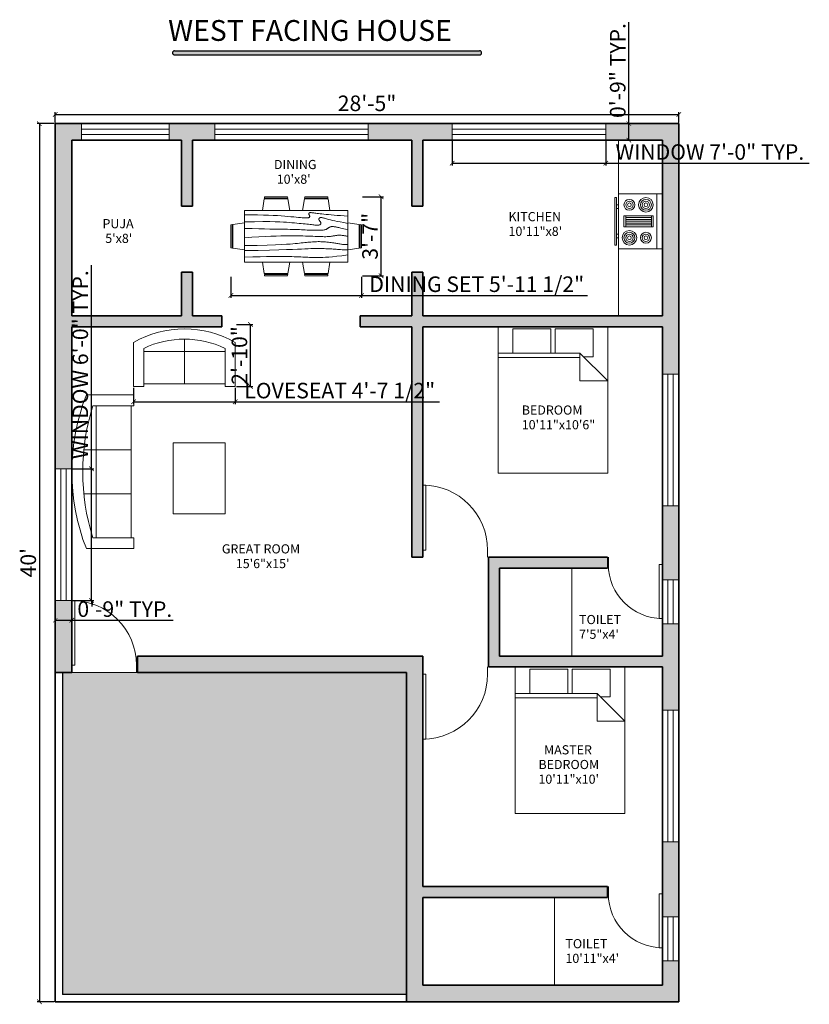
# Model space of a CAD drawing. Units: inches. Extents: x 3799 to 20199, y 1682 to 8087.
# Tile 30 of 30: x 19767 to 20199, y 6806 to 7344. Entities that reach past the tile are written whole.
import ezdxf

# ---------------------------------------------------------------- set-up
doc = ezdxf.new("R2010")
doc.units = ezdxf.units.IN
for name, color, linetype, lineweight in [('A-ANNO-DIMS', 2, 'Continuous', 18), ('A-ANNO-TITL', 7, 'Continuous', 25), ('A-AREA-IDEN', 7, 'Continuous', 18), ('A-DOOR', 3, 'Continuous', 18), ('A-EQPM', 9, 'Continuous', 18), ('A-FLOR-CASE', 32, 'Continuous', 18), ('A-FLOR-FIXT', 9, 'Continuous', 18), ('A-FURN', 8, 'Continuous', 18), ('A-GLAZ', 152, 'Continuous', 18), ('A-WALL', 7, 'Continuous', 35), ('A-WALL-PATT', 252, 'Continuous', 13), ('C-PROP', 7, 'Continuous', 25), ('L-PAVE', 253, 'Continuous', 13)]:
    doc.layers.add(name, color=color, linetype=linetype, lineweight=lineweight)
doc.styles.get("Standard").update_dxf_attribs({"font": 'arial.ttf'})
doc.dimstyles.new('ISO-25', dxfattribs={"dimtxt": 8.5, "dimasz": 2.5, "dimexe": 1.25, "dimexo": 0.625, "dimtad": 1, "dimdec": 0, "dimlunit": 3, "dimtxsty": 'Standard', "dimblk": 'ARCHTICK', "dimcen": 2.5, "dimadec": 0, "dimazin": 0, "dimtfac": 1, "dimtdec": 0, "dimtmove": 0, "dimatfit": 3, "dimfxl": 1, "dimarcsym": 0})

# ---------------------------------------------------------------- blocks, each defined once
blk = doc.blocks.new('*U49')
for p, q in [((0, 0), (0, -100)), ((900, 0), (900, -100))]:
    blk.add_line(p, q)
blk.add_lwpolyline([(0, 0), (0, 900), (43.75, 900), (43.75, 0)], close=True)
blk.add_arc((0, 0), 900, 0, 90)
blk = doc.blocks.new('*U215')
for p, q in [((0, 0), (0, 100)), ((900, 0), (900, 100))]:
    blk.add_line(p, q)
blk.add_lwpolyline([(0, 0), (0, -900), (43.75, -900), (43.75, 0)], close=True)
blk.add_arc((0, 0), 900, 270, 0)
blk = doc.blocks.new('*U216')
for p, q in [((-750, 0), (-750, 100)), ((0, 0), (0, 100))]:
    blk.add_line(p, q)
blk.add_lwpolyline([(0, 0), (0, -750), (-43.75, -750), (-43.75, 0)], close=True)
blk.add_arc((0, 0), 750, 180, 270)
blk = doc.blocks.new('Dining Set - 36 x 72 in.')
for p, q in [((-22, 27.5), (-22.1562, 26.50042)), ((-22, 27.5), (-6, 27.5)), ((-5.8437, 26.49966), (-6, 27.5)), ((6, 27.5), (5.8438, 26.50042)), ((6, 27.5), (22, 27.5)), ((22.1563, 26.49966), (22, 27.5)), ((-22.2343, 26.00059), (-23.4847, 17.99762)), ((-22.2304, 26), (-5.7608, 26)), ((-5.8416, 26.5), (-22.1534, 26.5)), ((-4.5152, 17.99762), (-5.7655, 25.99926)), ((5.7657, 26.00059), (4.5153, 17.99762)), ((5.7696, 26), (22.2392, 26)), ((22.1584, 26.5), (5.8466, 26.5)), ((23.4848, 17.99762), (22.2345, 25.99926)), ((36, 18), (-36, 18)), ((-36, 18), (-36, -18)), ((36, -18), (36, 18)), ((-45.5, 8), (-44.5004, 8.15617)), ((-45.5, 8), (-45.5, -8)), ((-44.5, -8.15843), (-44.5, 8.15338)), ((-44.0006, 8.23428), (-35.9976, 9.48474)), ((-44, 8.23041), (-44, -8.23915)), ((44.0006, 8.23428), (35.9976, 9.48474)), ((44, 8.23041), (44, -8.23915)), ((44.5, -8.15843), (44.5, 8.15338)), ((45.5, 8), (44.5005, 8.15617)), ((45.5, 8), (45.5, -8)), ((-44.4997, -8.15631), (-45.5, -8)), ((-35.9976, -9.48476), (-43.9993, -8.2345)), ((35.9976, -9.48476), (43.9993, -8.2345)), ((44.4997, -8.15631), (45.5, -8)), ((-36, -18), (36, -18)), ((-22.2343, -26.0006), (-23.4847, -17.99762)), ((-4.5152, -17.99762), (-5.7655, -25.99928)), ((5.7657, -26.0006), (4.5153, -17.99762)), ((23.4848, -17.99762), (22.2345, -25.99928)), ((-22.2304, -26), (-5.7608, -26)), ((-22, -27.5), (-22.1562, -26.50044)), ((-5.8416, -26.5), (-22.1534, -26.5)), ((-5.8437, -26.49967), (-6, -27.5)), ((5.7696, -26), (22.2392, -26)), ((6, -27.5), (5.8438, -26.50044)), ((22.1584, -26.5), (5.8466, -26.5)), ((22.1563, -26.49967), (22, -27.5)), ((-22, -27.5), (-6, -27.5)), ((6, -27.5), (22, -27.5))]:
    blk.add_line(p, q)
for points in [[(-36, 15), (-31.1772, 14.97754), (-26.8079, 14.91406), (-22.8538, 14.81543), (-19.276, 14.6875), (-16.0362, 14.53613), (-13.0957, 14.36718), (-10.4159, 14.18652), (-7.9583, 14), (-5.6904, 13.81315), (-3.6035, 13.63021), (-1.6954, 13.45508), (0.0365, 13.29166), (1.5945, 13.14388), (2.9811, 13.01562), (4.1988, 12.9108), (5.25, 12.83333), (6.1393, 12.78613), (6.8802, 12.76823), (7.4883, 12.77767), (7.9792, 12.8125), (8.3685, 12.87077), (8.6719, 12.95052), (8.9049, 13.0498), (9.0833, 13.16666), (9.2205, 13.29899), (9.3216, 13.44401), (9.3895, 13.59879), (9.4271, 13.76041), (9.4373, 13.92594), (9.4232, 14.09245), (9.3875, 14.257), (9.3333, 14.41666), (9.2638, 14.56917), (9.1836, 14.71484), (9.0975, 14.85465), (9.0104, 14.98958), (8.9272, 15.1206), (8.8529, 15.2487), (8.7922, 15.37483), (8.75, 15.5), (8.7305, 15.62467), (8.7344, 15.74739), (8.7617, 15.86621), (8.8125, 15.97916), (8.8867, 16.08431), (8.9844, 16.17968), (9.1055, 16.26334), (9.25, 16.33333), (9.4189, 16.38802), (9.6172, 16.42708), (9.8506, 16.45052), (10.125, 16.45833), (10.4463, 16.45052), (10.8203, 16.42708), (11.2529, 16.38802), (11.75, 16.33333), (12.3184, 16.26318), (12.9694, 16.17838), (13.7151, 16.07991), (14.5677, 15.96875), (15.5395, 15.84586), (16.6426, 15.71224), (17.8893, 15.56884), (19.2917, 15.41666), (20.859, 15.25667), (22.5879, 15.08984), (24.4721, 14.91715), (26.5052, 14.73958), (28.6809, 14.5581), (30.9929, 14.3737), (33.4347, 14.18733), (36, 14)], [(-36, 10), (-28.9766, 10.14274), (-23.1725, 10.20442), (-18.4241, 10.19775), (-14.5677, 10.13541), (-11.4399, 10.03011), (-8.877, 9.89453), (-6.7154, 9.74137), (-4.7917, 9.58333), (-2.9698, 9.43082), (-1.2246, 9.28515), (0.4415, 9.14534), (2.026, 9.01041), (3.5266, 8.87939), (4.9408, 8.7513), (6.266, 8.62516), (7.5, 8.5), (8.6411, 8.37549), (9.6914, 8.2539), (10.6538, 8.13818), (11.5312, 8.03125), (12.3267, 7.93603), (13.043, 7.85547), (13.6831, 7.79248), (14.25, 7.75), (14.7471, 7.7303), (15.1797, 7.73307), (15.5537, 7.75732), (15.875, 7.80208), (16.1494, 7.86637), (16.3828, 7.94922), (16.5811, 8.04964), (16.75, 8.16666), (16.8944, 8.29915), (17.0143, 8.44531), (17.1089, 8.60319), (17.1771, 8.77083), (17.218, 8.94629), (17.2305, 9.1276), (17.2137, 9.31282), (17.1667, 9.5), (17.0895, 9.6875), (16.987, 9.875), (16.8649, 10.0625), (16.7292, 10.25), (16.5856, 10.4375), (16.4401, 10.625), (16.2985, 10.8125), (16.1667, 11), (16.05, 11.18733), (15.9518, 11.3737), (15.8752, 11.5581), (15.8229, 11.73958), (15.798, 11.91715), (15.8034, 12.08984), (15.842, 12.25667), (15.9167, 12.41666), (16.0295, 12.56836), (16.1784, 12.70833), (16.3605, 12.83268), (16.5729, 12.9375), (16.8127, 13.01888), (17.0768, 13.07291), (17.3625, 13.0957), (17.6667, 13.08333), (17.9894, 13.03312), (18.3418, 12.94726), (18.7382, 12.82918), (19.1927, 12.68229), (19.7195, 12.51001), (20.3327, 12.31575), (21.0465, 12.10294), (21.875, 11.875), (22.8357, 11.63354), (23.959, 11.37304), (25.2786, 11.08618), (26.8282, 10.76562), (28.6414, 10.40405), (30.752, 9.99414), (33.1936, 9.52856), (36, 9)], [(-36, 5.5), (-30.7157, 5.3348), (-26.069, 5.20963), (-21.9946, 5.11767), (-18.4271, 5.05208), (-15.3009, 5.00602), (-12.5508, 4.97265), (-10.1112, 4.94515), (-7.9167, 4.91666), (-5.909, 4.88167), (-4.0586, 4.83984), (-2.3429, 4.79215), (-0.7396, 4.73958), (0.7739, 4.6831), (2.22, 4.6237), (3.6213, 4.56233), (5, 4.5), (6.373, 4.43782), (7.7344, 4.3776), (9.0723, 4.32129), (10.375, 4.27083), (11.6309, 4.22819), (12.8281, 4.19531), (13.9551, 4.17415), (15, 4.16666), (15.954, 4.17448), (16.819, 4.19791), (17.6001, 4.23698), (18.3021, 4.29166), (18.9299, 4.36198), (19.4883, 4.44791), (19.9823, 4.54948), (20.4167, 4.66666), (20.7969, 4.79899), (21.1302, 4.94401), (21.4245, 5.09879), (21.6875, 5.26041), (21.9271, 5.42594), (22.1511, 5.59245), (22.3672, 5.757), (22.5834, 5.91666), (22.8065, 6.06868), (23.0404, 6.21093), (23.2879, 6.34147), (23.5521, 6.45833), (23.8358, 6.55957), (24.142, 6.64323), (24.4735, 6.70735), (24.8334, 6.75), (25.2235, 6.76969), (25.642, 6.76692), (26.0858, 6.74267), (26.5521, 6.69791), (27.0379, 6.63362), (27.5404, 6.55078), (28.0565, 6.45036), (28.5834, 6.33333), (29.1242, 6.19987), (29.7071, 6.04687), (30.3661, 5.87044), (31.1354, 5.66666), (32.0493, 5.43164), (33.142, 5.16146), (34.4475, 4.85221), (36, 4.5)], [(-36, -1), (-30.7915, -0.6591), (-26.0195, -0.38216), (-21.6519, -0.16284), (-17.6563, 0.00521), (-14.0005, 0.12833), (-10.6523, 0.21289), (-7.5796, 0.26522), (-4.75, 0.29166), (-2.134, 0.29793), (0.2878, 0.28711), (2.5317, 0.26163), (4.6146, 0.22396), (6.5529, 0.17651), (8.3633, 0.12174), (10.0623, 0.06209), (11.6667, 0), (13.1899, -0.06201), (14.6341, -0.1211), (15.9982, -0.17432), (17.2813, -0.21875), (18.4823, -0.25147), (19.6003, -0.26953), (20.6343, -0.27002), (21.5834, -0.25), (22.4481, -0.20768), (23.2357, -0.14584), (23.9549, -0.06836), (24.6146, 0.02083), (25.2235, 0.11784), (25.7904, 0.21875), (26.3241, 0.31966), (26.8334, 0.41666), (27.3265, 0.50618), (27.8099, 0.58593), (28.2894, 0.65397), (28.7709, 0.70833), (29.2601, 0.74707), (29.763, 0.76823), (30.2855, 0.76985), (30.8334, 0.75), (31.4088, 0.70784), (31.9994, 0.64713), (32.589, 0.57275), (33.1615, 0.48958), (33.7008, 0.4025), (34.1908, 0.3164), (34.6153, 0.23616), (34.9584, 0.16666), (35.2099, 0.11165), (35.3848, 0.07031), (35.504, 0.04069), (35.5886, 0.02083), (35.6594, 0.00879), (35.7377, 0.0026), (35.8442, 0.00032), (36, 0)], [(-36, -6.5), (-27.1843, -6.31267), (-20.084, -6.1263), (-14.469, -5.9419), (-10.1094, -5.76042), (-6.7752, -5.58285), (-4.2363, -5.41016), (-2.2629, -5.24333), (-0.625, -5.08334), (0.8708, -4.93099), (2.2715, -4.78646), (3.5872, -4.64974), (4.8281, -4.52084), (6.0046, -4.39974), (7.127, -4.28646), (8.2053, -4.18099), (9.25, -4.08334), (10.2705, -3.99382), (11.2734, -3.91407), (12.2647, -3.84603), (13.25, -3.79167), (14.2354, -3.75293), (15.2266, -3.73177), (16.2295, -3.73015), (17.25, -3.75), (18.2912, -3.79248), (19.3451, -3.85547), (20.4009, -3.93604), (21.4479, -4.03125), (22.4754, -4.13819), (23.4727, -4.25391), (24.4289, -4.37549), (25.3334, -4.5), (26.1785, -4.62492), (26.9694, -4.74935), (27.7145, -4.87281), (28.4219, -4.99479), (29.1, -5.11483), (29.7572, -5.23242), (30.4016, -5.34709), (31.0417, -5.45834), (31.6837, -5.56437), (32.3262, -5.65821), (32.9658, -5.73153), (33.599, -5.77604), (34.2224, -5.78345), (34.8327, -5.74545), (35.4264, -5.65373), (36, -5.5)], [(-36, -10), (-26.4022, -9.81299), (-18.4675, -9.62891), (-11.9839, -9.45069), (-6.7396, -9.28125), (-2.5226, -9.12354), (0.8789, -8.98047), (3.6769, -8.85498), (6.0833, -8.75), (8.2767, -8.66765), (10.3021, -8.60677), (12.1712, -8.56543), (13.8958, -8.54167), (15.4876, -8.53353), (16.9583, -8.53907), (18.3197, -8.55632), (19.5834, -8.58334), (20.7616, -8.61841), (21.8685, -8.66081), (22.9188, -8.71004), (23.9271, -8.76563), (24.9081, -8.82707), (25.8763, -8.89388), (26.8465, -8.96558), (27.8334, -9.04167), (28.8474, -9.12118), (29.8828, -9.20117), (30.93, -9.27824), (31.9792, -9.34896), (33.0205, -9.40991), (34.0443, -9.45768), (35.0407, -9.48885), (36, -9.5)], [(-36, -14.5), (-30.0881, -14.33513), (-25.0332, -14.21224), (-20.7312, -14.12647), (-17.0781, -14.07292), (-13.97, -14.04671), (-11.3027, -14.04297), (-8.9724, -14.05681), (-6.875, -14.08334), (-4.9224, -14.11833), (-3.0905, -14.16016), (-1.3709, -14.20785), (0.2448, -14.26042), (1.7647, -14.3169), (3.1973, -14.3763), (4.5507, -14.43767), (5.8333, -14.5), (7.0554, -14.5621), (8.235, -14.62175), (9.3922, -14.67652), (10.5469, -14.72396), (11.7192, -14.76164), (12.929, -14.78711), (14.1965, -14.79794), (15.5417, -14.79167), (16.9933, -14.76424), (18.6152, -14.70508), (20.4804, -14.60197), (22.6615, -14.44271), (25.2312, -14.21509), (28.2624, -13.9069), (31.8277, -13.50594), (36, -13)]]:
    blk.add_lwpolyline(points)
blk = doc.blocks.new('Bed - Queen')
for p, q in [((0, -80.00003), (0, 0)), ((0, 0), (59.99999, 0)), ((59.99999, 0), (59.99999, -80.00003)), ((7.99999, -1.2), (28.79998, -1.2)), ((7.99999, -14.4), (7.99999, -1.2)), ((28.79998, -1.2), (28.79998, -14.4)), ((31.19999, -1.2), (51.99999, -1.2)), ((31.19999, -14.4), (31.19999, -1.2)), ((51.99999, -1.2), (51.99999, -16.4)), ((0, -14.4), (44.8, -14.4)), ((59.99999, -29.6), (44.8, -14.4)), ((44.8, -14.4), (44.8, -29.6)), ((44.8, -16.8), (0, -16.8)), ((51.99999, -16.4), (46.79936, -16.4)), ((44.8, -29.6), (59.99999, -29.6)), ((59.99999, -80.00003), (0, -80.00003))]:
    blk.add_line(p, q)
blk = doc.blocks.new('Range-Oven - 30 in top')
for p, q in [((0, -3), (30, -3)), ((12, -6), (18, -6)), ((13, -20), (13, -6)), ((14, -6), (14, -20)), ((15, -20), (15, -6)), ((16, -6), (16, -20)), ((17, -20), (17, -6)), ((18, -20), (12, -20)), ((6, -24), (6, -25)), ((8, -25), (8, -24)), ((22, -25), (22, -24)), ((24, -24), (24, -25))]:
    blk.add_line(p, q)
for points in [[(0, -24), (0, 0), (30, 0), (30, -24)], [(12, -21), (12, -5), (18, -5), (18, -21)], [(2, -26), (2, -25), (28, -25), (28, -26)]]:
    blk.add_lwpolyline(points, close=True)
for centre, radius in [((6, -9), 4), ((6, -9), 3), ((6, -9), 2), ((6, -9), 1), ((24, -9), 3), ((24, -9), 2), ((24, -9), 1), ((6, -18), 3), ((6, -18), 2), ((24, -18), 4), ((24, -18), 3), ((24, -18), 2), ((6, -18), 1), ((24, -18), 1)]:
    blk.add_circle(centre, radius)
blk = doc.blocks.new('Sofa - Roundback 7 ft.')
for p, q in [((-12.00002, -32.4421), (-12.00003, -6.5971)), ((11.99997, -32.4421), (11.99998, -6.5971)), ((-36.000027, -34), (-36.000027, -11.4696)), ((-35.999844, -13.3819), (35.9998, -13.3819)), ((35.99998, -34), (35.99998, -11.4696)), ((-36.000027, -32.4421), (35.99998, -32.4421))]:
    blk.add_line(p, q)
for points in [[(-36.000027, -34), (-42.000027, -34), (-42.000027, -8)], [(41.99998, -8), (41.99998, -34), (35.99998, -34)]]:
    blk.add_lwpolyline(points)
for centre, radius, start, end in [((0, -114.25), 114.25, 68.43141, 111.5686), ((-0.00001, -127.1968), 121.1968, 72.72033, 107.2797)]:
    blk.add_arc(centre, radius, start, end)
blk = doc.blocks.new('Sofa - Roundback Loveseat 5 ft.')
for p, q in [((-24, -33.99998), (-24, -11.46958)), ((0, -32.44198), (0, -5.99998)), ((24.00004, -33.99998), (24.00004, -11.46958)), ((-23.9998, -13.38178), (23.99986, -13.38178)), ((-24, -32.44198), (24.00004, -32.44198))]:
    blk.add_line(p, q)
for points in [[(-24, -33.99998), (-30, -33.99998), (-30, -7.99998)], [(30.00004, -7.99998), (30.00004, -33.99998), (24.00004, -33.99998)]]:
    blk.add_lwpolyline(points)
for centre, radius, start, end in [((0, -60.24998), 60.24998, 60.13715, 119.8628), ((0, -61.38438), 55.38444, 64.32083, 115.6792)]:
    blk.add_arc(centre, radius, start, end)
blk = doc.blocks.new('_ArchTick')
at = {"color": 0, "linetype": 'ByBlock', "const_width": 0.15}
blk.add_lwpolyline([(-0.5, -0.5), (0.5, 0.5)], dxfattribs=at)
blk = doc.blocks.new('*D217')
at = {"layer": 'A-ANNO-DIMS', "color": 0, "lineweight": -2, "transparency": 16777216}
for p, q in [((19786.54, 7287.57), (19786.54, 7293.26)), ((20127.54, 7287.57), (20127.54, 7293.26)), ((19786.54, 7292.01), (20127.54, 7292.01))]:
    blk.add_line(p, q, dxfattribs=at)
at = {"layer": 'Defpoints', "color": 0, "transparency": 16777216}
for p in [(20127.54, 7292.01), (19786.54, 7286.95), (20127.54, 7286.95)]:
    blk.add_point(p, dxfattribs=at)
at = {"layer": 'A-ANNO-DIMS', "color": 0, "lineweight": -2, "transparency": 16777216, "xscale": 2.5, "yscale": 2.5, "zscale": 2.5, "rotation": 180}
blk.add_blockref('_ArchTick', (19786.54, 7292.01), dxfattribs=at)
at = {"layer": 'A-ANNO-DIMS', "color": 0, "lineweight": -2, "transparency": 16777216, "xscale": 2.5, "yscale": 2.5, "zscale": 2.5}
blk.add_blockref('_ArchTick', (20127.54, 7292.01), dxfattribs=at)
at = {"layer": 'A-ANNO-DIMS', "color": 0, "transparency": 16777216, "insert": (19957.04, 7296.97), "char_height": 8.5, "attachment_point": 5}
blk.add_mtext('28\'-5"', dxfattribs=at)
blk = doc.blocks.new('*D218')
at = {"layer": 'A-ANNO-DIMS', "color": 0, "lineweight": -2, "transparency": 16777216}
for p, q in [((19785.92, 7286.95), (19776.58, 7286.95)), ((19777.83, 7286.95), (19777.83, 6806.95)), ((19785.92, 6806.95), (19776.58, 6806.95))]:
    blk.add_line(p, q, dxfattribs=at)
at = {"layer": 'Defpoints', "color": 0, "transparency": 16777216}
for p in [(19786.54, 7286.95), (19777.83, 6806.95), (19786.54, 6806.95)]:
    blk.add_point(p, dxfattribs=at)
at = {"layer": 'A-ANNO-DIMS', "color": 0, "lineweight": -2, "transparency": 16777216, "xscale": 2.5, "yscale": 2.5, "zscale": 2.5}
for p, rotation in [((19777.83, 7286.95), 90), ((19777.83, 6806.95), 270)]:
    blk.add_blockref('_ArchTick', p, dxfattribs=dict(at, rotation=rotation))
at = {"layer": 'A-ANNO-DIMS', "color": 0, "transparency": 16777216, "insert": (19772.87, 7046.95), "char_height": 8.5, "attachment_point": 5, "rotation": 90}
blk.add_mtext("40'", dxfattribs=at)
blk = doc.blocks.new('WIN-24IN-9IN-FRAME')
for p, q in [((0, 24), (9, 24)), ((3, 0), (3, 24)), ((6, 0), (6, 24)), ((0, 0), (9, 0))]:
    blk.add_line(p, q)
blk = doc.blocks.new('WIN-48IN-9IN-FRAME')
for p, q in [((0, 0), (0, 9)), ((48, 6), (0, 6)), ((48, 0), (48, 9)), ((48, 3), (0, 3))]:
    blk.add_line(p, q)
blk = doc.blocks.new('WIN-84IN-9IN-FRAME')
for p, q in [((0, 0), (0, 9)), ((0, 6), (84, 6)), ((84, 0), (84, 9)), ((0, 3), (84, 3))]:
    blk.add_line(p, q)
blk = doc.blocks.new('WIN-72IN-9IN-FRAME')
for p, q in [((0, 72), (9, 72)), ((3, 72), (3, 0)), ((6, 72), (6, 0)), ((0, 0), (9, 0))]:
    blk.add_line(p, q)
blk = doc.blocks.new('*D282')
at = {"layer": 'A-ANNO-DIMS', "color": 0, "lineweight": -2, "transparency": 16777216}
for p, q in [((19829.38, 7142.62), (19829.38, 7133.66)), ((19884.97, 7142.62), (19884.97, 7133.66)), ((19829.38, 7134.91), (19884.97, 7134.91)), ((19884.97, 7134.91), (19996.73, 7134.91))]:
    blk.add_line(p, q, dxfattribs=at)
at = {"layer": 'Defpoints', "color": 0, "transparency": 16777216}
for p in [(19829.38, 7143.25), (19884.97, 7143.25), (19884.97, 7134.91)]:
    blk.add_point(p, dxfattribs=at)
at = {"layer": 'A-ANNO-DIMS', "color": 0, "lineweight": -2, "transparency": 16777216, "xscale": 2.5, "yscale": 2.5, "zscale": 2.5, "rotation": 180}
blk.add_blockref('_ArchTick', (19829.38, 7134.91), dxfattribs=at)
at = {"layer": 'A-ANNO-DIMS', "color": 0, "lineweight": -2, "transparency": 16777216, "xscale": 2.5, "yscale": 2.5, "zscale": 2.5}
blk.add_blockref('_ArchTick', (19884.97, 7134.91), dxfattribs=at)
at = {"layer": 'A-ANNO-DIMS', "color": 0, "transparency": 16777216, "insert": (19942.1, 7139.93), "char_height": 8.5, "attachment_point": 5}
blk.add_mtext('LOVESEAT 4\'-7 1/2"', dxfattribs=at)
blk = doc.blocks.new('*D283')
at = {"layer": 'A-ANNO-DIMS', "color": 0, "lineweight": -2, "transparency": 16777216}
for p, q in [((19885.59, 7177.21), (19894.55, 7177.21)), ((19893.3, 7143.25), (19893.3, 7177.21)), ((19885.59, 7143.25), (19894.55, 7143.25))]:
    blk.add_line(p, q, dxfattribs=at)
at = {"layer": 'Defpoints', "color": 0, "transparency": 16777216}
for p in [(19884.97, 7177.21), (19893.3, 7177.21), (19884.97, 7143.25)]:
    blk.add_point(p, dxfattribs=at)
at = {"layer": 'A-ANNO-DIMS', "color": 0, "lineweight": -2, "transparency": 16777216, "xscale": 2.5, "yscale": 2.5, "zscale": 2.5}
for p, rotation in [((19893.3, 7177.21), 90), ((19893.3, 7143.25), 270)]:
    blk.add_blockref('_ArchTick', p, dxfattribs=dict(at, rotation=rotation))
at = {"layer": 'A-ANNO-DIMS', "color": 0, "transparency": 16777216, "insert": (19888.34, 7160.23), "char_height": 8.5, "attachment_point": 5, "rotation": 90}
blk.add_mtext('2\'-10"', dxfattribs=at)
blk = doc.blocks.new('*D296')
at = {"layer": 'A-ANNO-DIMS', "color": 0, "lineweight": -2, "transparency": 16777216}
for p, q in [((19882.55, 7203.16), (19882.55, 7191.82)), ((19954, 7203.16), (19954, 7191.82)), ((19882.55, 7193.07), (19954, 7193.07)), ((19954, 7193.07), (20077.58, 7193.07))]:
    blk.add_line(p, q, dxfattribs=at)
at = {"layer": 'Defpoints', "color": 0, "transparency": 16777216}
for p in [(19882.55, 7203.78), (19954, 7203.78), (19954, 7193.07)]:
    blk.add_point(p, dxfattribs=at)
at = {"layer": 'A-ANNO-DIMS', "color": 0, "lineweight": -2, "transparency": 16777216, "xscale": 2.5, "yscale": 2.5, "zscale": 2.5, "rotation": 180}
blk.add_blockref('_ArchTick', (19882.55, 7193.07), dxfattribs=at)
at = {"layer": 'A-ANNO-DIMS', "color": 0, "lineweight": -2, "transparency": 16777216, "xscale": 2.5, "yscale": 2.5, "zscale": 2.5}
blk.add_blockref('_ArchTick', (19954, 7193.07), dxfattribs=at)
at = {"layer": 'A-ANNO-DIMS', "color": 0, "transparency": 16777216, "insert": (20017.04, 7198.09), "char_height": 8.5, "attachment_point": 5}
blk.add_mtext('DINING SET 5\'-11 1/2"', dxfattribs=at)
blk = doc.blocks.new('*D297')
at = {"layer": 'A-ANNO-DIMS', "color": 0, "lineweight": -2, "transparency": 16777216}
for p, q in [((19954.62, 7246.97), (19965.97, 7246.97)), ((19964.72, 7203.78), (19964.72, 7246.97)), ((19954.62, 7203.78), (19965.97, 7203.78))]:
    blk.add_line(p, q, dxfattribs=at)
at = {"layer": 'Defpoints', "color": 0, "transparency": 16777216}
for p in [(19954, 7246.97), (19964.72, 7246.97), (19954, 7203.78)]:
    blk.add_point(p, dxfattribs=at)
at = {"layer": 'A-ANNO-DIMS', "color": 0, "lineweight": -2, "transparency": 16777216, "xscale": 2.5, "yscale": 2.5, "zscale": 2.5}
for p, rotation in [((19964.72, 7246.97), 90), ((19964.72, 7203.78), 270)]:
    blk.add_blockref('_ArchTick', p, dxfattribs=dict(at, rotation=rotation))
at = {"layer": 'A-ANNO-DIMS', "color": 0, "transparency": 16777216, "insert": (19959.75, 7225.38), "char_height": 8.5, "attachment_point": 5, "rotation": 90}
blk.add_mtext('3\'-7"', dxfattribs=at)
blk = doc.blocks.new('*D328')
at = {"layer": 'A-ANNO-DIMS', "color": 0, "lineweight": -2, "transparency": 16777216}
for p, q in [((19806.34, 7098.32), (19806.34, 7209.63)), ((19796.17, 7098.32), (19807.59, 7098.32)), ((19806.34, 7026.32), (19806.34, 7098.32)), ((19796.17, 7026.32), (19807.59, 7026.32))]:
    blk.add_line(p, q, dxfattribs=at)
at = {"layer": 'Defpoints', "color": 0, "transparency": 16777216}
for p in [(19795.54, 7098.32), (19806.34, 7098.32), (19795.54, 7026.32)]:
    blk.add_point(p, dxfattribs=at)
at = {"layer": 'A-ANNO-DIMS', "color": 0, "lineweight": -2, "transparency": 16777216, "xscale": 2.5, "yscale": 2.5, "zscale": 2.5}
for p, rotation in [((19806.34, 7098.32), 90), ((19806.34, 7026.32), 270)]:
    blk.add_blockref('_ArchTick', p, dxfattribs=dict(at, rotation=rotation))
at = {"layer": 'A-ANNO-DIMS', "color": 0, "transparency": 16777216, "insert": (19801.32, 7155.22), "char_height": 8.5, "attachment_point": 5, "rotation": 90}
blk.add_mtext('WINDOW 6\'-0" TYP.', dxfattribs=at)
blk = doc.blocks.new('*D329')
at = {"layer": 'A-ANNO-DIMS', "color": 0, "lineweight": -2, "transparency": 16777216}
for p, q in [((19786.54, 7025.69), (19786.54, 7014.27)), ((19795.54, 7025.69), (19795.54, 7014.27)), ((19786.54, 7015.52), (19795.54, 7015.52)), ((19795.54, 7015.52), (19851.1, 7015.52))]:
    blk.add_line(p, q, dxfattribs=at)
at = {"layer": 'Defpoints', "color": 0, "transparency": 16777216}
for p in [(19786.54, 7026.32), (19795.54, 7026.32), (19795.54, 7015.52)]:
    blk.add_point(p, dxfattribs=at)
at = {"layer": 'A-ANNO-DIMS', "color": 0, "lineweight": -2, "transparency": 16777216, "xscale": 2.5, "yscale": 2.5, "zscale": 2.5, "rotation": 180}
blk.add_blockref('_ArchTick', (19786.54, 7015.52), dxfattribs=at)
at = {"layer": 'A-ANNO-DIMS', "color": 0, "lineweight": -2, "transparency": 16777216, "xscale": 2.5, "yscale": 2.5, "zscale": 2.5}
blk.add_blockref('_ArchTick', (19795.54, 7015.52), dxfattribs=at)
at = {"layer": 'A-ANNO-DIMS', "color": 0, "transparency": 16777216, "insert": (19824.57, 7020.48), "char_height": 8.5, "attachment_point": 5}
blk.add_mtext('0\'-9" TYP.', dxfattribs=at)
blk = doc.blocks.new('*D340')
at = {"layer": 'A-ANNO-DIMS', "color": 0, "lineweight": -2, "transparency": 16777216}
for p, q in [((20003.6, 7277.32), (20003.6, 7264.1)), ((20087.6, 7277.32), (20087.6, 7264.1)), ((20003.6, 7265.35), (20087.6, 7265.35)), ((20087.6, 7265.35), (20198.91, 7265.35))]:
    blk.add_line(p, q, dxfattribs=at)
at = {"layer": 'Defpoints', "color": 0, "transparency": 16777216}
for p in [(20003.6, 7277.95), (20087.6, 7277.95), (20087.6, 7265.35)]:
    blk.add_point(p, dxfattribs=at)
at = {"layer": 'A-ANNO-DIMS', "color": 0, "lineweight": -2, "transparency": 16777216, "xscale": 2.5, "yscale": 2.5, "zscale": 2.5, "rotation": 180}
blk.add_blockref('_ArchTick', (20003.6, 7265.35), dxfattribs=at)
at = {"layer": 'A-ANNO-DIMS', "color": 0, "lineweight": -2, "transparency": 16777216, "xscale": 2.5, "yscale": 2.5, "zscale": 2.5}
blk.add_blockref('_ArchTick', (20087.6, 7265.35), dxfattribs=at)
at = {"layer": 'A-ANNO-DIMS', "color": 0, "transparency": 16777216, "insert": (20144.51, 7270.37), "char_height": 8.5, "attachment_point": 5}
blk.add_mtext('WINDOW 7\'-0" TYP.', dxfattribs=at)
blk = doc.blocks.new('*D341')
at = {"layer": 'A-ANNO-DIMS', "color": 0, "lineweight": -2, "transparency": 16777216}
for p, q in [((20100.2, 7286.95), (20100.2, 7342.51)), ((20088.23, 7286.95), (20101.45, 7286.95)), ((20100.2, 7277.95), (20100.2, 7286.95)), ((20088.23, 7277.95), (20101.45, 7277.95))]:
    blk.add_line(p, q, dxfattribs=at)
at = {"layer": 'Defpoints', "color": 0, "transparency": 16777216}
for p in [(20087.6, 7286.95), (20100.2, 7286.95), (20087.6, 7277.95)]:
    blk.add_point(p, dxfattribs=at)
at = {"layer": 'A-ANNO-DIMS', "color": 0, "lineweight": -2, "transparency": 16777216, "xscale": 2.5, "yscale": 2.5, "zscale": 2.5}
for p, rotation in [((20100.2, 7286.95), 90), ((20100.2, 7277.95), 270)]:
    blk.add_blockref('_ArchTick', p, dxfattribs=dict(at, rotation=rotation))
at = {"layer": 'A-ANNO-DIMS', "color": 0, "transparency": 16777216, "insert": (20095.24, 7315.98), "char_height": 8.5, "attachment_point": 5, "rotation": 90}
blk.add_mtext('0\'-9" TYP.', dxfattribs=at)

msp = doc.modelspace()

# ---------------------------------------------------------------- hatches: boundary and pattern name
at = {"layer": 'A-ANNO-TITL'}
h = msp.add_hatch(color=256, dxfattribs=at)
h.dxf.hatch_style = 1
h.paths.add_polyline_path([(20018.56, 7326.79), (19851.73, 7326.79, 1), (19851.73, 7324.51), (20018.56, 7324.51, 1)])
at = {"layer": 'A-WALL-PATT'}
h = msp.add_hatch(color=256, dxfattribs=at)
h.dxf.hatch_style = 1
h.paths.add_polyline_path([(19795.54, 7277.95), (19800.83, 7277.95), (19800.83, 7286.95), (19786.54, 7286.95), (19786.54, 7098.32), (19795.54, 7098.32), (19795.54, 7175.95), (19877.69, 7175.95), (19877.69, 7181.95), (19861.54, 7181.95), (19861.54, 7205.82), (19855.54, 7205.82), (19855.54, 7181.95), (19795.54, 7181.95)])
h.paths.add_polyline_path([(19873.75, 7286.95), (19848.83, 7286.95), (19848.83, 7277.95), (19855.54, 7277.95), (19855.54, 7241.82), (19861.54, 7241.82), (19861.54, 7277.95), (19873.75, 7277.95)], flags=17)
h.paths.add_polyline_path([(20003.6, 7286.95), (19957.75, 7286.95), (19957.75, 7277.95), (19981.54, 7277.95), (19981.54, 7241.82), (19987.54, 7241.82), (19987.54, 7277.95), (20003.6, 7277.95)], flags=17)
h.paths.add_polyline_path([(20127.54, 7286.95), (20087.6, 7286.95), (20087.6, 7277.95), (20118.54, 7277.95), (20118.54, 7181.95), (19987.54, 7181.95), (19987.54, 7205.82), (19981.54, 7205.82), (19981.54, 7181.95), (19953.3, 7181.95), (19953.3, 7175.95), (19981.54, 7175.95), (19981.54, 7049.95), (19987.54, 7049.95), (19987.54, 7175.95), (20118.54, 7175.95), (20118.54, 7149.99), (20127.54, 7149.99)])
h.paths.add_polyline_path([(20127.54, 7077.99), (20118.54, 7077.99), (20118.54, 7049.95), (20118.54, 7037.51), (20127.54, 7037.51)])
h.paths.add_polyline_path([(20127.54, 7013.51), (20118.54, 7013.51), (20118.54, 6995.95), (20029.54, 6995.95), (20029.54, 7043.95), (20088.54, 7043.95), (20088.54, 7049.95), (20023.54, 7049.95), (20023.54, 7043.95), (20023.54, 6989.95), (20118.54, 6989.95), (20118.54, 6966.36), (20127.54, 6966.36)])
h.paths.add_polyline_path([(20127.54, 6894.36), (20118.54, 6894.36), (20118.54, 6853.34), (20127.54, 6853.34)], flags=17)
h.paths.add_polyline_path([(20088.54, 6869.95), (19987.54, 6869.95), (19987.54, 6995.95), (19831.54, 6995.95), (19831.54, 6986.95), (19978.54, 6986.95), (19978.54, 6806.95), (20127.54, 6806.95), (20127.54, 6829.34), (20118.54, 6829.34), (20118.54, 6815.95), (19987.54, 6815.95), (19987.54, 6863.95), (20088.54, 6863.95)])
h.paths.add_polyline_path([(19795.54, 7026.32), (19786.54, 7026.32), (19786.54, 6986.95), (19795.54, 6986.95)])
at = {"layer": 'L-PAVE'}
h = msp.add_hatch(color=256, dxfattribs=at)
h.dxf.hatch_style = 1
h.paths.add_polyline_path([(19978.54, 6986.95), (19831.54, 6986.95), (19795.54, 6986.95), (19790.54, 6986.95), (19790.54, 6810.95), (19978.54, 6810.95)])

# ---------------------------------------------------------------- linework, layer by layer
at = {"layer": 'A-ANNO-TITL'}
for p, q in [((19851.73, 7326.79), (20018.56, 7326.79)), ((19851.73, 7324.51), (20018.56, 7324.51))]:
    msp.add_line(p, q, dxfattribs=at)
for centre, start, end in [((19851.73, 7325.65), 90, 270), ((20018.56, 7325.65), 270, 90)]:
    msp.add_arc(centre, 1.14, start, end, dxfattribs=at)
at = {"layer": 'A-DOOR'}
msp.add_line((19795.54, 6986.95), (19831.54, 6986.95), dxfattribs=at)
at = {"layer": 'A-FLOR-CASE'}
msp.add_line((20094.54, 7277.95), (20094.54, 7181.95), dxfattribs=at)
at = {"layer": 'A-FLOR-FIXT'}
for p, q in [((20069.05, 7043.95), (20069.05, 6995.95)), ((20059.51, 6863.95), (20059.51, 6815.95))]:
    msp.add_line(p, q, dxfattribs=at)
at = {"layer": 'A-FURN'}
msp.add_lwpolyline([(19851.07, 7112.49), (19879.43, 7112.49), (19879.43, 7073.72), (19851.07, 7073.72)], close=True, dxfattribs=at)
at = {"layer": 'A-WALL'}
for p, q in [((19786.54, 6986.95), (19786.54, 7286.95)), ((19786.54, 7286.95), (20127.54, 7286.95)), ((20127.54, 7286.95), (20127.54, 6806.95)), ((19795.54, 7277.95), (19855.54, 7277.95)), ((19795.54, 7181.95), (19795.54, 7277.95)), ((19855.54, 7241.82), (19855.54, 7277.95)), ((19861.54, 7277.95), (19981.54, 7277.95)), ((19861.54, 7241.82), (19861.54, 7277.95)), ((19981.54, 7241.82), (19981.54, 7277.95)), ((19987.54, 7277.95), (20118.54, 7277.95)), ((19987.54, 7241.82), (19987.54, 7277.95)), ((20118.54, 7277.95), (20118.54, 7181.95)), ((19855.54, 7241.82), (19861.54, 7241.82)), ((19981.54, 7241.82), (19987.54, 7241.82)), ((19855.54, 7181.95), (19855.54, 7205.82)), ((19855.54, 7205.82), (19861.54, 7205.82)), ((19861.54, 7181.95), (19861.54, 7205.82)), ((19981.54, 7181.95), (19981.54, 7205.82)), ((19981.54, 7205.82), (19987.54, 7205.82)), ((19987.54, 7181.95), (19987.54, 7205.82)), ((19795.54, 7181.95), (19855.54, 7181.95)), ((19861.54, 7181.95), (19877.69, 7181.95)), ((19877.69, 7181.95), (19877.69, 7175.95)), ((19953.3, 7181.95), (19981.54, 7181.95)), ((19953.3, 7181.95), (19953.3, 7175.95)), ((19987.54, 7181.95), (20118.54, 7181.95)), ((19795.54, 6986.95), (19795.54, 7175.95)), ((19795.54, 7175.95), (19877.69, 7175.95)), ((19953.3, 7175.95), (19981.54, 7175.95)), ((19981.54, 7049.95), (19981.54, 7175.95)), ((19987.54, 7175.95), (20118.54, 7175.95)), ((19987.54, 7049.95), (19987.54, 7175.95)), ((20118.54, 7175.95), (20118.54, 7049.95)), ((19987.54, 7049.95), (19981.54, 7049.95)), ((20023.54, 7049.95), (20088.54, 7049.95)), ((20023.54, 7043.95), (20023.54, 7049.95)), ((20118.54, 7049.95), (20118.54, 6995.95)), ((20023.54, 7043.95), (20023.54, 6989.95)), ((20029.54, 7043.95), (20029.54, 6995.95)), ((20029.54, 7043.95), (20088.54, 7043.95)), ((19831.54, 6995.95), (19987.54, 6995.95)), ((19831.54, 6986.95), (19831.54, 6995.95)), ((19987.54, 6869.95), (19987.54, 6995.95)), ((20029.54, 6995.95), (20118.54, 6995.95)), ((19786.54, 6986.95), (19795.54, 6986.95)), ((19786.54, 6986.95), (19786.54, 6806.95)), ((19831.54, 6986.95), (19978.54, 6986.95)), ((19978.54, 6806.95), (19978.54, 6986.95)), ((20023.54, 6989.95), (20118.54, 6989.95)), ((20118.54, 6989.95), (20118.54, 6815.95)), ((19987.54, 6869.95), (20088.54, 6869.95)), ((20088.54, 6869.95), (20088.54, 6863.95)), ((19987.54, 6815.95), (19987.54, 6863.95)), ((19987.54, 6863.95), (20088.54, 6863.95)), ((20118.54, 6815.95), (19987.54, 6815.95)), ((20127.54, 6806.95), (19786.54, 6806.95))]:
    msp.add_line(p, q, dxfattribs=at)
at = {"layer": 'C-PROP'}
for p, q in [((20088.54, 7049.95), (20088.54, 7043.95)), ((19790.54, 6986.95), (19790.54, 6810.95)), ((19978.54, 6810.95), (19790.54, 6810.95))]:
    msp.add_line(p, q, dxfattribs=at)

# ---------------------------------------------------------------- block references
at = {"layer": 'A-DOOR', "xscale": 0.0393700787401575, "yscale": 0.0393700787401575, "zscale": 0.0393700787401575}
for name, p in [('*U49', (19987.54, 7053.88)), ('*U216', (20118.54, 7046.01)), ('*U49', (19795.54, 6990.88)), ('*U215', (19987.54, 6986.01)), ('*U216', (20118.54, 6866.01))]:
    msp.add_blockref(name, p, dxfattribs=at)
at = {"layer": 'A-EQPM', "rotation": 270}
msp.add_blockref('Range-Oven - 30 in top', (20118.54, 7248.58), dxfattribs=at)
at = {"layer": 'A-FURN'}
for name, p, xscale, yscale, zscale in [('Dining Set - 36 x 72 in.', (19918.27, 7225.38), 0.7851969363924316, 0.7851969363924316, 0.7851969363924316), ('Sofa - Roundback Loveseat 5 ft.', (19857.17, 7174.74), 0.9264126650425815, 0.9264126650425815, 0.9264126650425815)]:
    msp.add_blockref(name, p, dxfattribs=dict(at, xscale=xscale, yscale=yscale, zscale=zscale))
for p in [(20028.69, 7175.95), (20038.01, 6989.95)]:
    msp.add_blockref('Bed - Queen', p, dxfattribs=at)
at = {"layer": 'A-FURN', "rotation": 90}
msp.add_blockref('Sofa - Roundback 7 ft.', (19795.57, 7096.63), dxfattribs=at)
at = {"layer": 'A-GLAZ'}
for name, p in [('WIN-48IN-9IN-FRAME', (19800.83, 7277.95)), ('WIN-84IN-9IN-FRAME', (19873.74, 7277.95)), ('WIN-84IN-9IN-FRAME', (20003.6, 7277.95)), ('WIN-72IN-9IN-FRAME', (20118.54, 7077.99)), ('WIN-72IN-9IN-FRAME', (19786.54, 7026.32)), ('WIN-24IN-9IN-FRAME', (20118.54, 7013.51)), ('WIN-72IN-9IN-FRAME', (20118.54, 6894.36)), ('WIN-24IN-9IN-FRAME', (20118.54, 6829.34))]:
    msp.add_blockref(name, p, dxfattribs=at)

# ---------------------------------------------------------------- texts
at = {"layer": 'A-ANNO-TITL'}
msp.add_text('WEST FACING HOUSE', height=11.3809, rotation=0.0014, dxfattribs=at).set_placement((19848.28, 7332.19))
at = {"layer": 'A-AREA-IDEN'}
for s, p in [('DINING', (19906.13, 7262.12)), (" 10'x8'", (19906.13, 7254.09)), ('PUJA', (19812.35, 7229.79)), ('KITCHEN', (20034.4, 7233.63)), ('10\'11"x8\'', (20034.4, 7225.6)), (" 5'x8'", (19812.35, 7221.76)), ('BEDROOM', (20041.66, 7127.9)), ('10\'11"x10\'6"', (20041.66, 7119.87)), ('GREAT ROOM', (19877.64, 7052.02)), ('     15\'6"x15\'', (19877.64, 7043.99)), ('TOILET', (20073, 7013.38)), ('7\'5"x4\'', (20073, 7005.35)), ('  MASTER', (20050.77, 6942.18)), ('BEDROOM', (20050.77, 6934.15)), ('10\'11"x10\'', (20050.77, 6926.12)), ('TOILET', (20065.54, 6836.22)), ('10\'11"x4\'', (20065.54, 6828.19))]:
    msp.add_text(s, height=5, rotation=0.0014, dxfattribs=at).set_placement(p)

# ---------------------------------------------------------------- dimensions: what is measured, and where the dimension line sits
at = {"layer": 'A-ANNO-DIMS'}
for base, p1, p2, text, picture, middle in [((20100.2, 7286.95), (20087.6, 7277.95), (20087.6, 7286.95), '<> TYP.', '*D341', (20095.24, 7315.98)), ((19806.34, 7098.32), (19795.54, 7026.32), (19795.54, 7098.32), 'WINDOW <> TYP.', '*D328', (19801.32, 7155.22))]:
    dim = msp.add_linear_dim(base=base, p1=p1, p2=p2, angle=90, text=text, dimstyle='ISO-25', override={"dimdec": 1, "dimlfac": 1, "dimrnd": 0, "dimzin": 1, "dimdsep": 46, "dimlunit": 4, "dimfrac": 2}, dxfattribs=at)
    dim.commit()
    dim.dimension.update_dxf_attribs({"geometry": picture, "text_midpoint": middle})
dim = msp.add_linear_dim(base=(20127.54, 7292.01), p1=(19786.54, 7286.95), p2=(20127.54, 7286.95), dimstyle='ISO-25', override={"dimclrd": 0, "dimclre": 0, "dimclrt": 0}, dxfattribs=at)
dim.commit()
dim.dimension.update_dxf_attribs({"geometry": '*D217', "text_midpoint": (19957.04, 7296.97)})
for base, p1, p2, override, picture, middle in [((19777.83, 6806.95), (19786.54, 7286.95), (19786.54, 6806.95), {"dimclrd": 0, "dimclre": 0, "dimclrt": 0}, '*D218', (19772.87, 7046.95)), ((19964.72, 7246.97), (19954, 7203.78), (19954, 7246.97), {"dimdec": 1, "dimlfac": 1, "dimrnd": 0, "dimzin": 1, "dimdsep": 46, "dimlunit": 4, "dimfrac": 2}, '*D297', (19959.75, 7225.38)), ((19893.3, 7177.21), (19884.97, 7143.25), (19884.97, 7177.21), {"dimdec": 1, "dimlfac": 1, "dimrnd": 0, "dimzin": 1, "dimdsep": 46, "dimlunit": 4, "dimfrac": 2}, '*D283', (19888.34, 7160.23))]:
    dim = msp.add_linear_dim(base=base, p1=p1, p2=p2, angle=90, dimstyle='ISO-25', override=override, dxfattribs=at)
    dim.commit()
    dim.dimension.update_dxf_attribs({"geometry": picture, "text_midpoint": middle})
for base, p1, p2, text, picture, middle in [((20087.6, 7265.35), (20003.6, 7277.95), (20087.6, 7277.95), 'WINDOW <> TYP.', '*D340', (20144.51, 7270.37)), ((19953.9997, 7193.0655), (19882.5468, 7203.7834), (19953.9997, 7203.7834), 'DINING SET <>', '*D296', (20017.0421, 7198.0854)), ((19884.97, 7134.91), (19829.38, 7143.25), (19884.97, 7143.25), 'LOVESEAT <>', '*D282', (19942.1, 7139.93)), ((19795.54, 7015.52), (19786.54, 7026.32), (19795.54, 7026.32), '<> TYP.', '*D329', (19824.57, 7020.48))]:
    dim = msp.add_linear_dim(base=base, p1=p1, p2=p2, text=text, dimstyle='ISO-25', override={"dimdec": 1, "dimlfac": 1, "dimrnd": 0, "dimzin": 1, "dimdsep": 46, "dimlunit": 4, "dimfrac": 2}, dxfattribs=at)
    dim.commit()
    dim.dimension.update_dxf_attribs({"geometry": picture, "text_midpoint": middle})

doc.saveas('drawing.dxf')
